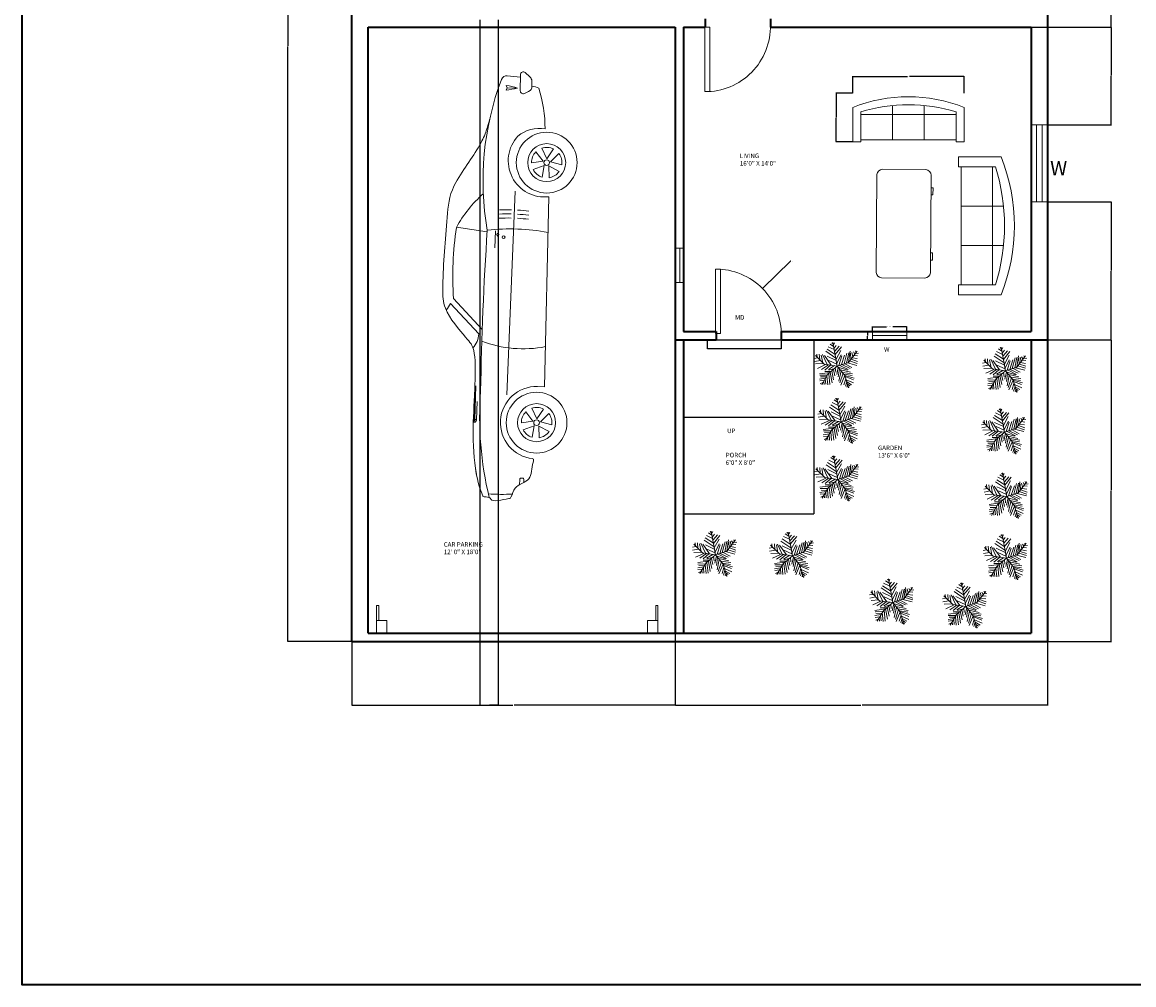
# Model space of a CAD drawing. Units: inches. Extents: x 65 to 1274, y 42 to 1041.
# Tile 1 of 6: x 65 to 678, y 42 to 573. Entities that reach past the tile are written whole.
import ezdxf

# ---------------------------------------------------------------- set-up
doc = ezdxf.new("R2010")
doc.units = ezdxf.units.IN
for name, color, linetype, lineweight in [('A-ANNO-DIMS', 2, 'Continuous', 18), ('A-AREA-IDEN', 7, 'Continuous', 18), ('A-DOOR', 3, 'Continuous', 18), ('A-EQPM-VEHI', 8, 'Continuous', 13), ('A-FLOR-STRS', 2, 'Continuous', 25), ('A-FURN', 8, 'Continuous', 18), ('A-GLAZ', 4, 'Continuous', 18), ('A-WALL', 7, 'Continuous', 35), ('C-SITE', 8, 'Continuous', 18), ('L-PLNT', 94, 'Continuous', 13), ('Text', 7, 'Continuous', 18), ('Title Block', 7, 'Continuous', 35)]:
    doc.layers.add(name, color=color, linetype=linetype, lineweight=lineweight)
doc.styles.get("Standard").update_dxf_attribs({"font": 'arial.ttf'})
doc.dimstyles.get("Standard").update_dxf_attribs({"dimtxt": 0.18, "dimasz": 0.18, "dimexe": 0.18, "dimexo": 0.0625, "dimgap": 0.09, "dimtad": 0, "dimtih": 1, "dimtoh": 1, "dimdec": 4, "dimzin": 0, "dimdsep": 46, "dimtxsty": 'Standard', "dimcen": 0.09, "dimadec": 0, "dimazin": 0, "dimtfac": 1, "dimtdec": 4, "dimtofl": 0, "dimtmove": 0, "dimatfit": 3, "dimfxl": 1, "dimtolj": 1, "dimtzin": 0, "dimarcsym": 0})

# ---------------------------------------------------------------- blocks, each defined once
blk = doc.blocks.new('*U2')
for p, q in [((72.93, 40.23), (85.8, 53.18)), ((75, 38.82), (88.08, 51.97)), ((119.39, 51.91), (117.92, 38.32)), ((50.13, 41.06), (34.31, 40.98)), ((43.26, 39.85), (35.15, 39.78)), ((35.3, 40.46), (50.13, 40.62)), ((111.09, 34.73), (118.48, 34.64)), ((46.65, 26.83), (136.29, 26.77)), ((180.37, 26.17), (187.51, 26.41)), ((7.45, 19.78), (9.74, 19.8)), ((179.3, 24.35), (180.25, 22.49)), ((182.62, 21.14), (184.91, 21.28)), ((186.68, 22.17), (188.51, 24.37)), ((9.76, 17.93), (8.53, 17.92)), ((10.37, 19.19), (10.38, 18.56)), ((50.87, 13.52), (50.91, 10.52))]:
    blk.add_line(p, q)
for points in [[(35.31, 39.93), (35.3, 40.27, 0.269532), (35.14, 40.54), (34.38, 40.96, 0.575383), (34.15, 40.83), (34.15, 40.49, 0.269532), (34.32, 40.22), (35.08, 39.79, 0.575383)], [(34.64, 20.05), (35.56, 14.97), (39.5, 18.31, 0.199906)], [(148.99, 20.05), (149.91, 14.97), (153.85, 18.31, 0.199906)], [(28.49, 15.1), (33.61, 14.4), (31.65, 19.18, 0.199906)], [(41.25, 15.74), (36.7, 13.3), (41.09, 10.58, 0.199906)], [(142.85, 15.1), (147.96, 14.4), (146.01, 19.18, 0.199906)], [(155.6, 15.74), (151.06, 13.3), (155.45, 10.58, 0.199906)], [(31.31, 7.72), (33.55, 12.37), (28.4, 11.99, 0.199906)], [(39.19, 8.12), (35.46, 11.69), (34.23, 6.67, 0.199906)], [(145.66, 7.72), (147.9, 12.37), (142.75, 11.99, 0.199906)], [(153.54, 8.12), (149.81, 11.69), (148.59, 6.67, 0.199906)]]:
    blk.add_lwpolyline(points, format="xyb", close=True)
for points in [[(181.58, 27.46), (181.53, 31.95), (180.48, 32.43)], [(181.58, 27.46), (181.53, 31.95), (182.57, 32.45)], [(50.91, 10.52), (134.38, 11.83)]]:
    blk.add_lwpolyline(points)
for centre, radius in [((115.89, 31.01), 0.619), ((34.98, 13.35), 13.35), ((149.33, 13.35), 13.35), ((34.98, 13.35), 8.35), ((149.33, 13.35), 8.35), ((34.98, 13.35), 1.25), ((149.33, 13.35), 1.25)]:
    blk.add_circle(centre, radius)
for centre, radius, start, end in [((114.6, 105.09), 59.37, 237.6103, 240.9785), ((103.45, -95), 147.78, 83.8163, 95.9705), ((95.51, 3.91), 53.61, 43.2748, 63.5665), ((20.53, -3.15), 43.06, 98.5304, 116.112), ((73.29, 50.49), 10.26, 230.424, 268.0085), ((145.17, -84.88), 125.99, 71.5283, 102.1242), ((42.18, -111.35), 149.91, 87.8393, 105.8096), ((80.1, -1364.13), 1402.96, 88.42296, 91.3179), ((118.31, 22.51), 51.16, 161.4307, 193.2363), ((25.66, 24.94), 94.01, 351.8279, 8.1674), ((184.3, 32.25), 2.49, 357.932, 71.5283), ((79.16, 30.11), 76.3, 177.5773, 185.5205), ((45.64, 26.83), 78.76, 0.852, 4.6556), ((47.43, 26.85), 78.76, 0.852, 4.6556), ((49.23, 26.87), 78.76, 0.852, 4.6556), ((150.1, 14.36), 15.92, 49.2263, 189.1528), ((216.26, 37.76), 36.17, 188.4683, 196.5315), ((146.68, 36.98), 36.17, 344.7432, 352.8063), ((116.55, 34.7), 70.29, 353.1942, 357.932), ((34.98, 13.35), 15.9, 0.6373, 176.3412), ((45.64, 26.83), 78.76, 355.2644, 358.8633), ((47.43, 26.85), 78.76, 355.2644, 358.8633), ((49.23, 26.87), 78.76, 355.2644, 358.8633), ((149.4, 16.55), 14.84, 352.7285, 41.6613), ((180.41, 24.92), 1.25, 91.939, 207.109), ((187.55, 25.16), 1.25, 320.1683, 91.939), ((9.75, 19.18), 0.623, 0.6373, 90.6373), ((182.47, 23.63), 2.49, 207.109, 273.4677), ((114.25, 37.03), 70.29, 344.3985, 346.9385), ((184.76, 23.76), 2.49, 273.4677, 320.1683), ((9.76, 18.55), 0.623, 270.6373, 0.6373), ((162.47, 70.82), 56.18, 271.6865, 290.2774)]:
    blk.add_arc(centre, radius, start, end)
blk.add_ellipse((116.89, 33.59), major_axis=(-0.63, -0.007), ratio=0.610043)
for points, knots in [([(11.39, 38.92), (18.06, 40.19), (30.91, 42.01), (64.77, 40.11), (70.25, 44.91), (82.35, 56.38), (99.18, 57.3), (116.06, 56.35), (133.04, 55.87), (145.24, 49.87), (153.62, 43.8), (161.17, 40.68), (164.92, 39.73), (167.29, 39.15)], [18.629823, 18.629823, 18.629823, 18.629823, 19.527405, 20.700571, 21.107983, 21.608568, 21.92336, 23.151359, 23.716171, 23.908743, 24.77794, 24.943072, 25.187755, 25.187755, 25.187755, 25.187755]), ([(19.11, 14.36), (18.99, 14.21), (18.5, 13.81), (15.35, 15), (9.19, 13.94), (7.26, 22.22), (3.01, 22.66), (1.32, 23.61), (0.64, 26.92), (-0.96, 31.49), (1.54, 32.64), (1.5, 34.06), (1.49, 34.8), (1.49, 35.06), (1.52, 35.3), (1.58, 35.51)], [16.815853, 16.815853, 16.815853, 16.815853, 16.838212, 16.885395, 17.18439, 17.479846, 17.654423, 17.670693, 17.696923, 18.016358, 18.052739, 18.140805, 18.140805, 18.140805, 18.172382, 18.172382, 18.172382, 18.172382])]:
    blk.add_open_spline(points, degree=3, knots=knots)
blk = doc.blocks.new('*U4')
for p, q in [((-10.186, 53.64), (-13.084, 55.962)), ((0, 0), (-10.5, 57)), ((-9.099, 51.782), (-6.563, 55.962)), ((-48.585, 21.131), (-49.309, 29.026)), ((-43.513, 28.561), (-42.427, 15.558)), ((-35.544, 28.097), (-24.314, 3.947)), ((-3.665, 19.273), (-27.574, 35.527)), ((-5.114, 28.097), (-24.676, 40.636)), ((-7.288, 39.707), (-21.778, 46.673)), ((-8.737, 47.138), (-17.069, 52.711)), ((-7.65, 43.423), (-2.578, 49.46)), ((-5.839, 35.992), (4.667, 48.067)), ((-5.114, 27.632), (10.463, 46.673)), ((-2.941, 16.486), (8.652, 37.85)), ((16.259, 5.805), (23.142, 31.348)), ((22.055, 7.198), (27.489, 32.277)), ((27, 9), (48, 36)), ((27.127, 9.056), (31.112, 35.992)), ((31.836, 30.883), (32.561, 16.486)), ((35.096, 32.741), (37.27, 22.524)), ((38.719, 34.134), (41.979, 28.561)), ((43.791, 29.954), (51.036, 30.883)), ((44.153, 36.456), (45.239, 32.741)), ((-47.498, 19.737), (-55.83, 18.344)), ((-40.615, 13.7), (-55.105, 10.913)), ((-31.5, 4.5), (-52.5, 25.5)), ((-33.37, 6.269), (-52.207, 5.34)), ((-28.299, 3.483), (-47.86, -5.805)), ((-38.442, 26.239), (-34.819, 7.663)), ((-21.416, 3.018), (-38.079, -8.128)), ((0, 0), (-31.5, 4.5)), ((-14.533, 2.09), (-30.834, 25.31)), ((-15.982, 2.09), (-30.11, -9.521)), ((-24.314, 23.917), (-2.941, 13.7)), ((0, 0), (-22.5, -19.5)), ((-6.563, 1.161), (-21.416, -8.128)), ((-20.691, 13.7), (-1.129, 4.876)), ((-1.129, 6.734), (9.014, 26.704)), ((0, 0), (27, 9)), ((0, 0), (18, -22.5)), ((3.942, 1.625), (11.187, 24.381)), ((6.478, 1.625), (26.04, -8.592)), ((10.101, 3.483), (17.708, 26.239)), ((11.187, 3.483), (30.749, -5.805)), ((18.07, 5.805), (35.096, -3.483)), ((24.229, 7.663), (46.688, 1.625)), ((29.662, 12.307), (48.137, 6.269)), ((33.285, 16.486), (48.862, 10.913)), ((36.183, 19.737), (48.137, 17.88)), ((40.53, 25.775), (48.862, 24.846)), ((-17.431, -15.094), (-42.789, -18.809)), ((-24.314, -21.596), (-42.427, -22.06)), ((-26.849, -26.24), (-40.253, -25.775)), ((-22.5, -19.5), (-37.5, -45)), ((-15.257, -12.772), (-30.11, -12.772)), ((-25.038, -23.918), (-22.865, -45.281)), ((-20.691, -18.345), (-17.793, -44.352)), ((-6.563, -5.805), (-19.967, -9.985)), ((-17.069, -15.094), (-12.721, -40.172)), ((-13.446, -11.378), (-8.737, -32.741)), ((-9.461, -8.592), (-6.201, -23.453)), ((-4.752, -3.483), (-3.665, -14.629)), ((2.493, -3.019), (-1.491, -20.202)), ((1.769, -2.555), (24.229, -9.521)), ((5.029, -6.27), (2.131, -25.775)), ((9.014, -11.378), (3.58, -35.992)), ((14.085, -16.951), (6.478, -40.172)), ((7.565, -9.056), (32.198, -14.629)), ((18.07, -22.524), (8.289, -45.745)), ((12.274, -15.094), (36.907, -18.809)), ((16.259, -19.738), (36.183, -22.989)), ((18, -22.5), (27, -52.5)), ((18.433, -22.524), (40.53, -29.026)), ((19.157, -25.311), (38.719, -33.206)), ((-28.299, -29.026), (-42.789, -31.348)), ((-30.834, -34.135), (-42.427, -35.528)), ((-34.457, -39.708), (-40.978, -42.494)), ((-32.646, -36.921), (-31.921, -44.352)), ((-29.023, -30.884), (-27.936, -43.887)), ((20.244, -30.419), (15.897, -44.816)), ((22.78, -37.85), (19.519, -48.532)), ((21.331, -32.741), (39.081, -40.636)), ((22.78, -38.314), (34.372, -44.816)), ((24.591, -45.745), (23.142, -50.854)), ((24.591, -43.423), (30.749, -47.603)), ((26.764, -49.925), (28.213, -50.854))]:
    blk.add_line(p, q)
blk = doc.blocks.new('Sofa - Roundback 7 ft.')
for p, q in [((-12.00002, -32.4421), (-12.00003, -6.5971)), ((11.99997, -32.4421), (11.99998, -6.5971)), ((-36.000027, -34), (-36.000027, -11.4696)), ((-35.999844, -13.3819), (35.9998, -13.3819)), ((35.99998, -34), (35.99998, -11.4696)), ((-36.000027, -32.4421), (35.99998, -32.4421))]:
    blk.add_line(p, q)
for points in [[(-36.000027, -34), (-42.000027, -34), (-42.000027, -8)], [(41.99998, -8), (41.99998, -34), (35.99998, -34)]]:
    blk.add_lwpolyline(points)
for centre, radius, start, end in [((0, -114.25), 114.25, 68.43141, 111.5686), ((-0.00001, -127.1968), 121.1968, 72.72033, 107.2797)]:
    blk.add_arc(centre, radius, start, end)
blk = doc.blocks.new('Desk - 30 x 60 in.')
for p, q in [((-26.999995, 0), (26.999995, 0)), ((-29.999995, -27), (-29.999995, -3)), ((29.999995, -3), (29.999995, -27)), ((26.999995, -30), (-26.999995, -30)), ((-20.000005, -30), (-20.000005, -31)), ((-16.000005, -31), (-16.000005, -30)), ((15.999995, -31), (15.999995, -30)), ((19.999995, -30), (19.999995, -31)), ((-20.000005, -31), (-16.000005, -31)), ((19.999995, -31), (15.999995, -31))]:
    blk.add_line(p, q)
for centre, start, end in [((-26.499995, -3.5), 98.1301, 171.8699), ((26.499995, -3.5), 8.130102, 81.8699), ((-26.499995, -26.5), 188.1301, 261.8699), ((26.499995, -26.5), 278.1301, 351.8699)]:
    blk.add_arc(centre, 3.535534, start, end)
blk = doc.blocks.new('WIN-43-DEEP-FRAME')
for p, q in [((9, 42.65), (0, 42.65)), ((0, 42.65), (0, 0)), ((3, 0), (3, 42.65)), ((6, 42.65), (6, 0)), ((9, 0), (9, 42.65)), ((0, 0), (9, 0))]:
    blk.add_line(p, q)
blk = doc.blocks.new('WIN-19-NARROW-FRAME')
for p, q in [((0, 4.5), (0, 0)), ((18.96, 4.5), (0, 4.5)), ((18.96, 2.5), (0, 2.5)), ((18.96, 2.5), (0, 2.5)), ((18.96, 2.5), (0, 2.5)), ((0, 0), (18.96, 0)), ((18.96, 0), (18.96, 4.5))]:
    blk.add_line(p, q)
blk = doc.blocks.new('DOOR-SINGLE-36')
blk.add_lwpolyline([(0.01, 1.25), (2.82, 1.25), (2.82, 36.75), (0.01, 36.75)], close=True)
blk.add_arc((0.35, 0.95), 35.9, 358.4887, 90.56146)
blk = doc.blocks.new('*D22')
at = {"layer": 'A-ANNO-DIMS', "color": 0, "lineweight": -2, "transparency": 16777216}
for p, q in [((534.07, 402.01), (534.07, 404.97)), ((553.03, 402.01), (553.03, 404.97)), ((534.25, 404.79), (541.83, 404.79)), ((552.85, 404.79), (545.27, 404.79))]:
    blk.add_line(p, q, dxfattribs=at)
at = {"layer": 'A-ANNO-DIMS', "color": 0, "transparency": 16777216}
for points in [[(534.25, 404.82), (534.25, 404.76), (534.07, 404.79)], [(552.85, 404.82), (552.85, 404.76), (553.03, 404.79)]]:
    blk.add_solid(points, dxfattribs=at)
at = {"layer": 'Defpoints', "color": 0, "transparency": 16777216}
for p in [(534.07, 401.94), (553.03, 404.79), (553.03, 401.94)]:
    blk.add_point(p, dxfattribs=at)
at = {"layer": 'A-ANNO-DIMS', "color": 0, "transparency": 16777216, "insert": (543.55, 404.79), "char_height": 0.18, "attachment_point": 5}
blk.add_mtext('\\A1;NARROW WINDOW 19 TYP.', dxfattribs=at)
blk = doc.blocks.new('*D23')
at = {"layer": 'A-ANNO-DIMS', "color": 0, "lineweight": -2, "transparency": 16777216}
for p, q in [((534.01, 401.94), (531.05, 401.94)), ((531.23, 401.76), (531.23, 399.88)), ((531.23, 397.62), (531.23, 399.51)), ((534.01, 397.44), (531.05, 397.44))]:
    blk.add_line(p, q, dxfattribs=at)
at = {"layer": 'A-ANNO-DIMS', "color": 0, "transparency": 16777216}
for points in [[(531.2, 401.76), (531.26, 401.76), (531.23, 401.94)], [(531.2, 397.62), (531.26, 397.62), (531.23, 397.44)]]:
    blk.add_solid(points, dxfattribs=at)
at = {"layer": 'Defpoints', "color": 0, "transparency": 16777216}
for p in [(531.23, 401.94), (534.07, 401.94), (534.07, 397.44)]:
    blk.add_point(p, dxfattribs=at)
at = {"layer": 'A-ANNO-DIMS', "color": 0, "transparency": 16777216, "insert": (531.23, 399.69), "char_height": 0.18, "attachment_point": 5}
blk.add_mtext('\\A1;5 TYP.', dxfattribs=at)
blk = doc.blocks.new('*D34')
at = {"layer": 'A-ANNO-DIMS', "color": 0, "lineweight": -2, "transparency": 16777216}
for p, q in [((523.15, 533.71), (523.15, 543.05)), ((523.33, 542.87), (553.31, 542.87)), ((584.45, 542.87), (554.47, 542.87)), ((584.63, 533.71), (584.63, 543.05))]:
    blk.add_line(p, q, dxfattribs=at)
at = {"layer": 'A-ANNO-DIMS', "color": 0, "transparency": 16777216}
for points in [[(523.33, 542.9), (523.33, 542.84), (523.15, 542.87)], [(584.45, 542.9), (584.45, 542.84), (584.63, 542.87)]]:
    blk.add_solid(points, dxfattribs=at)
at = {"layer": 'Defpoints', "color": 0, "transparency": 16777216}
for p in [(584.63, 542.87), (523.15, 533.65), (584.63, 533.65)]:
    blk.add_point(p, dxfattribs=at)
at = {"layer": 'A-ANNO-DIMS', "color": 0, "transparency": 16777216, "insert": (553.89, 542.87), "char_height": 0.18, "attachment_point": 5}
blk.add_mtext('\\A1;SOFA 61', dxfattribs=at)
blk = doc.blocks.new('*D35')
at = {"layer": 'A-ANNO-DIMS', "color": 0, "lineweight": -2, "transparency": 16777216}
for p, q in [((523.09, 533.65), (513.75, 533.65)), ((513.93, 533.47), (513.93, 520.41)), ((513.93, 506.99), (513.93, 520.05)), ((523.09, 506.81), (513.75, 506.81))]:
    blk.add_line(p, q, dxfattribs=at)
at = {"layer": 'A-ANNO-DIMS', "color": 0, "transparency": 16777216}
for points in [[(513.9, 533.47), (513.96, 533.47), (513.93, 533.65)], [(513.9, 506.99), (513.96, 506.99), (513.93, 506.81)]]:
    blk.add_solid(points, dxfattribs=at)
at = {"layer": 'Defpoints', "color": 0, "transparency": 16777216}
for p in [(513.93, 533.65), (523.15, 533.65), (523.15, 506.81)]:
    blk.add_point(p, dxfattribs=at)
at = {"layer": 'A-ANNO-DIMS', "color": 0, "transparency": 16777216, "insert": (513.93, 520.23), "char_height": 0.18, "attachment_point": 5}
blk.add_mtext('\\A1;27', dxfattribs=at)
blk = doc.blocks.new('*D53')
at = {"layer": 'A-ANNO-DIMS', "color": 0, "lineweight": -2, "transparency": 16777216}
for p, q in [((246.62, 888.1), (211.23, 888.1)), ((211.41, 887.92), (211.41, 559.78)), ((211.41, 231.28), (211.41, 559.42)), ((246.62, 231.1), (211.23, 231.1))]:
    blk.add_line(p, q, dxfattribs=at)
at = {"layer": 'A-ANNO-DIMS', "color": 0, "transparency": 16777216}
for points in [[(211.38, 887.92), (211.44, 887.92), (211.41, 888.1)], [(211.38, 231.28), (211.44, 231.28), (211.41, 231.1)]]:
    blk.add_solid(points, dxfattribs=at)
at = {"layer": 'Defpoints', "color": 0, "transparency": 16777216}
for p in [(211.41, 888.1), (246.69, 888.1), (246.69, 231.1)]:
    blk.add_point(p, dxfattribs=at)
at = {"layer": 'A-ANNO-DIMS', "color": 0, "transparency": 16777216, "insert": (211.41, 559.6), "char_height": 0.18, "attachment_point": 5}
blk.add_mtext('\\A1;657', dxfattribs=at)
blk = doc.blocks.new('*D54')
at = {"layer": 'A-ANNO-DIMS', "color": 0, "lineweight": -2, "transparency": 16777216}
for p, q in [((425.19, 235.54), (425.19, 195.72)), ((246.69, 231.04), (246.69, 195.72)), ((246.87, 195.9), (335.55, 195.9)), ((425.01, 195.9), (336.32, 195.9))]:
    blk.add_line(p, q, dxfattribs=at)
at = {"layer": 'A-ANNO-DIMS', "color": 0, "transparency": 16777216}
for points in [[(246.87, 195.93), (246.87, 195.87), (246.69, 195.9)], [(425.01, 195.93), (425.01, 195.87), (425.19, 195.9)]]:
    blk.add_solid(points, dxfattribs=at)
at = {"layer": 'Defpoints', "color": 0, "transparency": 16777216}
for p in [(425.19, 235.6), (246.69, 231.1), (425.19, 195.9)]:
    blk.add_point(p, dxfattribs=at)
at = {"layer": 'A-ANNO-DIMS', "color": 0, "transparency": 16777216, "insert": (335.94, 195.9), "char_height": 0.18, "attachment_point": 5}
blk.add_mtext('\\A1;178.5', dxfattribs=at)
blk = doc.blocks.new('*D55')
at = {"layer": 'A-ANNO-DIMS', "color": 0, "lineweight": -2, "transparency": 16777216}
for p, q in [((425.19, 235.54), (425.19, 195.72)), ((630.69, 231.04), (630.69, 195.72)), ((425.37, 195.9), (527.54, 195.9)), ((630.51, 195.9), (528.33, 195.9))]:
    blk.add_line(p, q, dxfattribs=at)
at = {"layer": 'A-ANNO-DIMS', "color": 0, "transparency": 16777216}
for points in [[(425.37, 195.93), (425.37, 195.87), (425.19, 195.9)], [(630.51, 195.93), (630.51, 195.87), (630.69, 195.9)]]:
    blk.add_solid(points, dxfattribs=at)
at = {"layer": 'Defpoints', "color": 0, "transparency": 16777216}
for p in [(425.19, 235.6), (630.69, 231.1), (630.69, 195.9)]:
    blk.add_point(p, dxfattribs=at)
at = {"layer": 'A-ANNO-DIMS', "color": 0, "transparency": 16777216, "insert": (527.94, 195.9), "char_height": 0.18, "attachment_point": 5}
blk.add_mtext('\\A1;205.5', dxfattribs=at)
blk = doc.blocks.new('*D56')
at = {"layer": 'A-ANNO-DIMS', "color": 0, "lineweight": -2, "transparency": 16777216}
for p, q in [((630.75, 397.6), (666.07, 397.6)), ((665.89, 397.42), (665.89, 314.53)), ((665.89, 231.28), (665.89, 314.17)), ((630.75, 231.1), (666.07, 231.1))]:
    blk.add_line(p, q, dxfattribs=at)
at = {"layer": 'A-ANNO-DIMS', "color": 0, "transparency": 16777216}
for points in [[(665.86, 397.42), (665.92, 397.42), (665.89, 397.6)], [(665.86, 231.28), (665.92, 231.28), (665.89, 231.1)]]:
    blk.add_solid(points, dxfattribs=at)
at = {"layer": 'Defpoints', "color": 0, "transparency": 16777216}
for p in [(630.69, 397.6), (665.89, 397.6), (630.69, 231.1)]:
    blk.add_point(p, dxfattribs=at)
at = {"layer": 'A-ANNO-DIMS', "color": 0, "transparency": 16777216, "insert": (665.89, 314.35), "char_height": 0.18, "attachment_point": 5}
blk.add_mtext('\\A1;166.5', dxfattribs=at)
blk = doc.blocks.new('*D57')
at = {"layer": 'A-ANNO-DIMS', "color": 0, "lineweight": -2, "transparency": 16777216}
for p, q in [((630.74, 473.63), (666.07, 473.63)), ((665.89, 473.45), (665.89, 435.8)), ((665.89, 397.78), (665.89, 435.43)), ((630.75, 397.6), (666.07, 397.6))]:
    blk.add_line(p, q, dxfattribs=at)
at = {"layer": 'A-ANNO-DIMS', "color": 0, "transparency": 16777216}
for points in [[(665.86, 473.45), (665.92, 473.45), (665.89, 473.63)], [(665.86, 397.78), (665.92, 397.78), (665.89, 397.6)]]:
    blk.add_solid(points, dxfattribs=at)
at = {"layer": 'Defpoints', "color": 0, "transparency": 16777216}
for p in [(630.68, 473.63), (665.89, 473.63), (630.69, 397.6)]:
    blk.add_point(p, dxfattribs=at)
at = {"layer": 'A-ANNO-DIMS', "color": 0, "transparency": 16777216, "insert": (665.89, 435.62), "char_height": 0.18, "attachment_point": 5}
blk.add_mtext('\\A1;76.03', dxfattribs=at)
blk = doc.blocks.new('*D58')
at = {"layer": 'A-ANNO-DIMS', "color": 0, "lineweight": -2, "transparency": 16777216}
for p, q in [((621.75, 570.1), (666.07, 570.1)), ((665.89, 569.92), (665.89, 543.37)), ((665.89, 516.46), (665.89, 543.01)), ((630.74, 516.28), (666.07, 516.28))]:
    blk.add_line(p, q, dxfattribs=at)
at = {"layer": 'A-ANNO-DIMS', "color": 0, "transparency": 16777216}
for points in [[(665.86, 569.92), (665.92, 569.92), (665.89, 570.1)], [(665.86, 516.46), (665.92, 516.46), (665.89, 516.28)]]:
    blk.add_solid(points, dxfattribs=at)
at = {"layer": 'Defpoints', "color": 0, "transparency": 16777216}
for p in [(621.69, 570.1), (665.89, 570.1), (630.68, 516.28)]:
    blk.add_point(p, dxfattribs=at)
at = {"layer": 'A-ANNO-DIMS', "color": 0, "transparency": 16777216, "insert": (665.89, 543.19), "char_height": 0.18, "attachment_point": 5}
blk.add_mtext('\\A1;53.82', dxfattribs=at)
blk = doc.blocks.new('*D59')
at = {"layer": 'A-ANNO-DIMS', "color": 0, "lineweight": -2, "transparency": 16777216}
for p, q in [((630.45, 629.46), (666.07, 629.46)), ((665.89, 629.28), (665.89, 599.96)), ((665.89, 570.28), (665.89, 599.6)), ((621.75, 570.1), (666.07, 570.1))]:
    blk.add_line(p, q, dxfattribs=at)
at = {"layer": 'A-ANNO-DIMS', "color": 0, "transparency": 16777216}
for points in [[(665.86, 629.28), (665.92, 629.28), (665.89, 629.46)], [(665.86, 570.28), (665.92, 570.28), (665.89, 570.1)]]:
    blk.add_solid(points, dxfattribs=at)
at = {"layer": 'Defpoints', "color": 0, "transparency": 16777216}
for p in [(630.39, 629.46), (665.89, 629.46), (621.69, 570.1)]:
    blk.add_point(p, dxfattribs=at)
at = {"layer": 'A-ANNO-DIMS', "color": 0, "transparency": 16777216, "insert": (665.89, 599.78), "char_height": 0.18, "attachment_point": 5}
blk.add_mtext('\\A1;59.36', dxfattribs=at)
blk = doc.blocks.new('*D63')
at = {"layer": 'A-ANNO-DIMS', "color": 0, "lineweight": -2, "transparency": 16777216}
for p, q in [((317.41, 574.21), (317.41, 195.72)), ((327.41, 574.21), (327.41, 195.72)), ((317.59, 195.9), (322.2, 195.9)), ((327.23, 195.9), (322.62, 195.9))]:
    blk.add_line(p, q, dxfattribs=at)
at = {"layer": 'A-ANNO-DIMS', "color": 0, "transparency": 16777216}
for points in [[(317.59, 195.93), (317.59, 195.87), (317.41, 195.9)], [(327.23, 195.93), (327.23, 195.87), (327.41, 195.9)]]:
    blk.add_solid(points, dxfattribs=at)
at = {"layer": 'Defpoints', "color": 0, "transparency": 16777216}
for p in [(317.41, 574.27), (327.41, 574.27), (327.41, 195.9)]:
    blk.add_point(p, dxfattribs=at)
at = {"layer": 'A-ANNO-DIMS', "color": 0, "transparency": 16777216, "insert": (322.41, 195.9), "char_height": 0.18, "attachment_point": 5}
blk.add_mtext('\\A1;10', dxfattribs=at)
blk = doc.blocks.new('*D80')
at = {"layer": 'A-ANNO-DIMS', "color": 0, "lineweight": -2, "transparency": 16777216}
for p, q in [((488.74, 440.95), (473.51, 425.97)), ((488.92, 440.95), (488.74, 440.95)), ((447.69, 400.67), (447.87, 400.67)), ((447.78, 400.58), (447.78, 400.76))]:
    blk.add_line(p, q, dxfattribs=at)
at = {"layer": 'A-ANNO-DIMS', "color": 0, "transparency": 16777216}
blk.add_solid([(473.49, 425.99), (473.53, 425.95), (473.38, 425.84)], dxfattribs=at)
at = {"layer": 'Defpoints', "color": 0, "transparency": 16777216}
for p in [(473.38, 425.84), (447.78, 400.67)]:
    blk.add_point(p, dxfattribs=at)
at = {"layer": 'A-ANNO-DIMS', "color": 0, "transparency": 16777216, "insert": (489.52, 440.95), "char_height": 0.18, "attachment_point": 5}
blk.add_mtext('\\A1;2X R35.9', dxfattribs=at)

msp = doc.modelspace()

# ---------------------------------------------------------------- linework, layer by layer
at = {"layer": 'A-FLOR-STRS'}
for p, q in [((501.6872, 397.6013), (501.6872, 301.6013)), ((429.7753, 354.8857), (501.5124, 354.8857)), ((429.6872, 301.6013), (501.6872, 301.6013))]:
    msp.add_line(p, q, dxfattribs=at)
msp.add_lwpolyline([(442.9783, 397.5386), (483.603, 397.5386), (483.603, 392.6497), (442.9783, 392.6497)], close=True, dxfattribs=at)
at = {"layer": 'A-WALL'}
for p, q in [((246.6872, 231.1013), (246.6872, 888.1013)), ((630.6872, 888.1013), (630.6872, 231.1013)), ((441.6872, 574.6013), (441.6872, 570.1013)), ((477.6872, 574.6013), (477.6872, 570.1013)), ((255.6872, 235.6013), (255.6872, 570.1013)), ((255.6872, 570.1013), (425.1872, 570.1013)), ((425.1872, 570.1013), (425.1872, 235.6013)), ((429.6872, 570.1013), (429.6872, 402.1013)), ((429.6872, 570.1013), (441.6872, 570.1013)), ((477.6872, 570.1013), (621.6872, 570.1013)), ((621.6872, 570.1013), (621.6872, 402.1013)), ((429.6872, 402.1013), (447.6872, 402.1013)), ((447.6872, 402.1013), (447.6872, 397.6013)), ((483.6872, 402.1013), (483.6872, 397.6013)), ((483.6872, 402.1013), (621.6872, 402.1013)), ((425.1872, 397.6013), (447.6872, 397.6013)), ((429.6872, 397.6013), (429.6872, 235.6013)), ((483.6872, 397.6013), (630.6872, 397.6013)), ((621.6872, 397.6013), (621.6872, 235.6013)), ((255.6872, 235.6013), (621.6872, 235.6013)), ((246.6872, 231.1013), (630.6872, 231.1013))]:
    msp.add_line(p, q, dxfattribs=at)
at = {"layer": 'C-SITE'}
for points in [[(260.3099, 242.6876), (261.4873, 242.6876), (261.4873, 250.9243), (260.3099, 250.9243)], [(414.4168, 242.6522), (415.5942, 242.6522), (415.5942, 250.8889), (414.4168, 250.8889)], [(260.3151, 235.6319), (265.9881, 235.6319), (265.9881, 242.6919), (260.3151, 242.6919)], [(409.907, 235.5904), (415.5799, 235.5904), (415.5799, 242.6504), (409.907, 242.6504)]]:
    msp.add_lwpolyline(points, close=True, dxfattribs=at)
at = {"layer": 'Title Block'}
msp.add_lwpolyline([(64.7421, 1041.286), (1273.976, 1041.286), (1273.976, 41.6396), (64.7421, 41.6396)], close=True, dxfattribs=at)

# ---------------------------------------------------------------- block references
at = {"layer": 'A-DOOR', "extrusion": (0, 0, -1), "zscale": -1, "rotation": 180}
msp.add_blockref('DOOR-SINGLE-36', (-441.4484, 571.3538), dxfattribs=at)
at = {"layer": 'A-DOOR'}
msp.add_blockref('DOOR-SINGLE-36', (447.4311, 399.721), dxfattribs=at)
at = {"layer": 'A-EQPM-VEHI', "xscale": 1.25592051339692, "yscale": 1.25592051339692, "zscale": 1.25592051339692, "rotation": 87.77464782570856}
msp.add_blockref('*U2', (363.7109, 307.2833), dxfattribs=at)
at = {"layer": 'A-FURN', "xscale": 0.7319422041462386, "yscale": 0.7319422041462386, "zscale": 0.7319422041462386}
msp.add_blockref('Sofa - Roundback 7 ft.', (553.8909, 531.7003), dxfattribs=at)
at = {"layer": 'A-FURN', "xscale": 0.9059646076568906, "yscale": 0.9059646076568906, "zscale": 0.9059646076568906, "rotation": 270}
msp.add_blockref('Sofa - Roundback 7 ft.', (612.3662, 460.4482), dxfattribs=at)
at = {"layer": 'A-FURN', "rotation": 89.4788228304995}
msp.add_blockref('Desk - 30 x 60 in.', (536.3009, 461.7761), dxfattribs=at)
at = {"layer": 'A-GLAZ'}
for name, p in [('WIN-43-DEEP-FRAME', (621.679, 473.63)), ('WIN-19-NARROW-FRAME', (534.072, 397.444))]:
    msp.add_blockref(name, p, dxfattribs=at)
at = {"layer": 'A-GLAZ', "rotation": 270.0000000000001}
msp.add_blockref('WIN-19-NARROW-FRAME', (425.2939, 448.0925), dxfattribs=at)
at = {"layer": 'L-PLNT', "xscale": 0.2291951906982327, "yscale": 0.2291951906982327, "zscale": 0.2291951906982327}
for p in [(514.6341, 383.0589), (607.5163, 380.4293), (516.7391, 352.2928), (606.99, 346.5078), (514.8972, 320.475), (608.3056, 311.0085), (447.4264, 278.8923), (489.8674, 278.3654), (607.964, 277.0482), (545.2252, 252.548), (585.5573, 250.4404)]:
    msp.add_blockref('*U4', p, dxfattribs=at)

# ---------------------------------------------------------------- texts
at = {"layer": 'A-AREA-IDEN', "char_height": 2.5, "attachment_point": 1}
for s, width, insert in [('LIVING\\P16\'0" X 14\'0"', 34.092354, (460.8644, 500.3589)), ('GARDEN\\P13\'6" X 6\'0"', 41.772781, (537.0915, 339.1867)), ('PORCH\\P6\'0" X 8\'0" ', 35.869474, (453.0775, 335.2071)), ('CAR PARKING\\P12\' 0" X 18\'0"', 49.264842, (297.4187, 285.9327))]:
    msp.add_mtext_dynamic_manual_height_columns(s, width=width, gutter_width=12.5, heights=[0], dxfattribs=dict(at, insert=insert))
at = {"layer": 'Text', "attachment_point": 1}
for s, width, gutter_width, insert, char_height in [('W', 96.254197, 39.1027, (632.1391, 496.1658), 7.8205), ('MD', 9.913037, 12.5, (458.2594, 411.1704), 2.5), ('W', 8.992402, 12.5, (540.4626, 393.4311), 2.5), ('UP', 17.758909, 12.5, (453.7808, 348.5619), 2.5)]:
    msp.add_mtext_dynamic_manual_height_columns(s, width=width, gutter_width=gutter_width, heights=[0], dxfattribs=dict(at, insert=insert, char_height=char_height))

# ---------------------------------------------------------------- dimensions: what is measured, and where the dimension line sits
at = {"layer": 'A-ANNO-DIMS'}
for base, p1, p2, override, picture, middle in [((211.4126, 888.1013), (246.6872, 231.1013), (246.6872, 888.1013), {"dimdec": 0, "dimlfac": 1, "dimrnd": 0, "dimzin": 0, "dimdsep": 46, "dimlunit": 2}, '*D53', (211.4126, 559.6013)), ((665.8872, 629.4605), (621.6872, 570.1013), (630.3914, 629.4605), {"dimdec": 2, "dimlfac": 1, "dimrnd": 0, "dimzin": 0, "dimdsep": 46, "dimlunit": 2}, '*D59', (665.8872, 599.7809)), ((665.8872, 570.1013), (630.679, 516.2787), (621.6872, 570.1013), {"dimdec": 2, "dimlfac": 1, "dimrnd": 0, "dimzin": 0, "dimdsep": 46, "dimlunit": 2}, '*D58', (665.8872, 543.19)), ((513.9269, 533.6522), (523.1493, 506.8143), (523.1493, 533.6522), {"dimdec": 0, "dimlfac": 1, "dimrnd": 0, "dimzin": 0, "dimdsep": 46, "dimlunit": 2}, '*D35', (513.9269, 520.2332)), ((665.8872, 473.6305), (630.6872, 397.6013), (630.679, 473.6305), {"dimdec": 2, "dimlfac": 1, "dimrnd": 0, "dimzin": 0, "dimdsep": 46, "dimlunit": 2}, '*D57', (665.8872, 435.6159)), ((665.8872, 397.6013), (630.6872, 231.1013), (630.6872, 397.6013), {"dimdec": 1, "dimlfac": 1, "dimrnd": 0, "dimzin": 0, "dimdsep": 46, "dimlunit": 2}, '*D56', (665.8872, 314.3513))]:
    dim = msp.add_linear_dim(base=base, p1=p1, p2=p2, angle=90, dimstyle='Standard', override=override, dxfattribs=at)
    dim.commit()
    dim.dimension.update_dxf_attribs({"geometry": picture, "text_midpoint": middle})
for base, p1, p2, override, picture, middle in [((327.4055, 195.9013), (317.4055, 574.2747), (327.4055, 574.2747), {"dimdec": 0, "dimlfac": 1, "dimrnd": 0, "dimzin": 0, "dimdsep": 46, "dimlunit": 2}, '*D63', (322.4055, 195.9013)), ((425.1872, 195.9013), (246.6872, 231.1013), (425.1872, 235.6013), {"dimdec": 1, "dimlfac": 1, "dimrnd": 0, "dimzin": 0, "dimdsep": 46, "dimlunit": 2}, '*D54', (335.9372, 195.9013)), ((630.6872, 195.9013), (425.1872, 235.6013), (630.6872, 231.1013), {"dimdec": 1, "dimlfac": 1, "dimrnd": 0, "dimzin": 0, "dimdsep": 46, "dimlunit": 2}, '*D55', (527.9372, 195.9013))]:
    dim = msp.add_linear_dim(base=base, p1=p1, p2=p2, dimstyle='Standard', override=override, dxfattribs=at)
    dim.commit()
    dim.dimension.update_dxf_attribs({"geometry": picture, "text_midpoint": middle})
for base, p1, p2, text, picture, middle in [((584.6325, 542.8746), (523.1493, 533.6522), (584.6325, 533.6522), 'SOFA <>', '*D34', (553.8909, 542.8746)), ((553.0295, 404.7877), (534.0717, 401.944), (553.0295, 401.944), 'NARROW WINDOW <> TYP.', '*D22', (543.5506, 404.7877))]:
    dim = msp.add_linear_dim(base=base, p1=p1, p2=p2, text=text, dimstyle='Standard', override={"dimdec": 0, "dimlfac": 1, "dimrnd": 0, "dimzin": 0, "dimdsep": 46, "dimlunit": 2}, dxfattribs=at)
    dim.commit()
    dim.dimension.update_dxf_attribs({"geometry": picture, "text_midpoint": middle})
dim = msp.add_radius_dim(center=(447.7828, 400.6684), mpoint=(473.3789, 425.8439), text='2X <>', dimstyle='Standard', override={"dimdec": 1, "dimlfac": 1, "dimrnd": 0, "dimzin": 0, "dimdsep": 46, "dimlunit": 2}, dxfattribs=at)
dim.commit()
dim.dimension.update_dxf_attribs({"geometry": '*D80', "text_midpoint": (489.5216, 440.9492), "dimtype": 164})
dim = msp.add_linear_dim(base=(531.2280250878, 401.9440128202), p1=(534.071696822, 397.4440128202), p2=(534.071696822, 401.9440128202), angle=90, text='<> TYP.', dimstyle='Standard', override={"dimdec": 0, "dimlfac": 1, "dimrnd": 0, "dimzin": 0, "dimdsep": 46, "dimlunit": 2}, dxfattribs=at)
dim.commit()
dim.dimension.update_dxf_attribs({"geometry": '*D23', "text_midpoint": (531.2280250878, 399.6940128202)})

doc.saveas('drawing.dxf')
